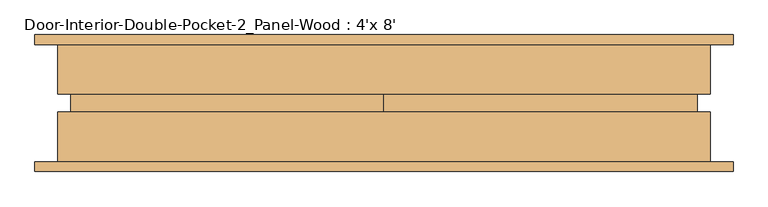
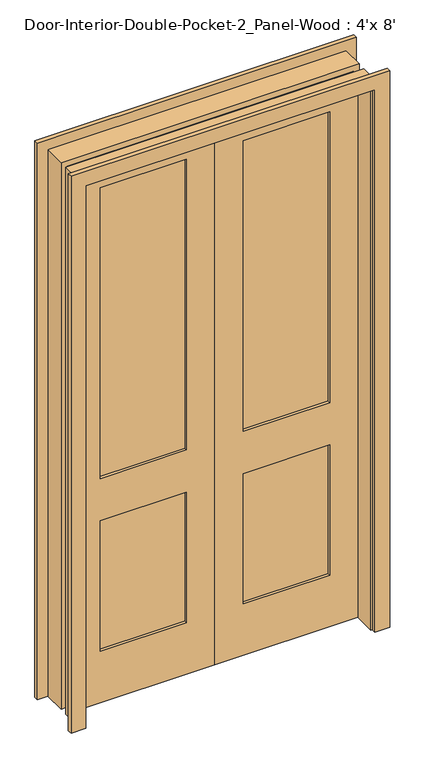
"""IFC4 building model written with IfcOpenShell, lengths in millimetres: door geometry, Door-Interior-Double-Pocket-2_Panel-Wood : 4'x 8'."""

from ifc_helpers import new_model, si_unit, frame, origin, place, context, project, spatial, polyline, outline, extrude, source, transform, mapped, element, save


def door_interior_double_pocket_2_panel_wood_4_x_8_12c354ae(model_context):
    return source(origin(), model_context, "Body", "SweptSolid", [
        extrude(outline(polyline([(0.0, 615.95), (0.0, 679.45), (2508.25, 679.45), (2508.25, -679.45), (0.0, -679.45), (0.0, -615.95), (2444.75, -615.95), (2444.75, 615.95), (0.0, 615.95)])), frame((0.0, 114.3, 0.0), z_axis=(0.0, 1.0, 0.0), x_axis=(0.0, 0.0, 1.0)), (0.0, 0.0, 1.0), 19.05),
        extrude(outline(polyline([(0.0, 615.95), (0.0, 679.45), (2508.25, 679.45), (2508.25, -679.45), (0.0, -679.45), (0.0, -615.95), (2444.75, -615.95), (2444.75, 615.95), (0.0, 615.95)])), frame((0.0, -133.35, 0.0), z_axis=(0.0, 1.0, 0.0), x_axis=(0.0, 0.0, 1.0)), (0.0, 0.0, 1.0), 19.05),
        extrude(outline(polyline([(2438.4, 0.0), (0.0, 0.0), (0.0, 609.6), (2438.4, 609.6), (2438.4, 0.0)]), holes=[polyline([(2319.3375, 120.65), (2319.3375, 488.95), (1009.65, 488.95), (1009.65, 120.65), (2319.3375, 120.65)]), polyline([(819.15, 120.65), (819.15, 488.95), (231.775, 488.95), (231.775, 120.65), (819.15, 120.65)])]), frame((0.0, -17.4625, 0.0), z_axis=(0.0, 1.0, 0.0), x_axis=(0.0, 0.0, 1.0)), (0.0, 0.0, 1.0), 34.925),
        extrude(outline(polyline([(488.95, -5.8208333), (120.65, -5.8208333), (120.65, 5.8208333), (488.95, 5.8208333), (488.95, -5.8208333)])), frame((0.0, 0.0, 1009.65), z_axis=(0.0, 0.0, 1.0), x_axis=(1.0, 0.0, 0.0)), (0.0, 0.0, 1.0), 1309.6875),
        extrude(outline(polyline([(488.95, -5.8208333), (120.65, -5.8208333), (120.65, 5.8208333), (488.95, 5.8208333), (488.95, -5.8208333)])), frame((0.0, 0.0, 231.775), z_axis=(0.0, 0.0, 1.0), x_axis=(1.0, 0.0, 0.0)), (0.0, 0.0, 1.0), 587.375),
        extrude(outline(polyline([(0.0, 635.0), (2463.8, 635.0), (2463.8, -635.0), (0.0, -635.0), (0.0, -609.6), (2438.4, -609.6), (2438.4, 609.6), (0.0, 609.6), (0.0, 635.0)])), frame((0.0, 17.4625, 0.0), z_axis=(0.0, 1.0, 0.0), x_axis=(0.0, 0.0, 1.0)), (0.0, 0.0, 1.0), 96.8375),
        extrude(outline(polyline([(0.0, 635.0), (2463.8, 635.0), (2463.8, -635.0), (0.0, -635.0), (0.0, -609.6), (2438.4, -609.6), (2438.4, 609.6), (0.0, 609.6), (0.0, 635.0)])), frame((0.0, -114.3, 0.0), z_axis=(0.0, 1.0, 0.0), x_axis=(0.0, 0.0, 1.0)), (0.0, 0.0, 1.0), 96.8375),
        extrude(outline(polyline([(2438.4, -609.6), (0.0, -609.6), (0.0, 0.0), (2438.4, 0.0), (2438.4, -609.6)]), holes=[polyline([(2319.3375, -488.95), (2319.3375, -120.65), (1009.65, -120.65), (1009.65, -488.95), (2319.3375, -488.95)]), polyline([(819.15, -488.95), (819.15, -120.65), (231.775, -120.65), (231.775, -488.95), (819.15, -488.95)])]), frame((0.0, -17.4625, 0.0), z_axis=(0.0, 1.0, 0.0), x_axis=(0.0, 0.0, 1.0)), (0.0, 0.0, 1.0), 34.925),
        extrude(outline(polyline([(-120.65, -5.8208333), (-488.95, -5.8208333), (-488.95, 5.8208333), (-120.65, 5.8208333), (-120.65, -5.8208333)])), frame((0.0, 0.0, 1009.65), z_axis=(0.0, 0.0, 1.0), x_axis=(1.0, 0.0, 0.0)), (0.0, 0.0, 1.0), 1309.6875),
        extrude(outline(polyline([(-120.65, -5.8208333), (-488.95, -5.8208333), (-488.95, 5.8208333), (-120.65, 5.8208333), (-120.65, -5.8208333)])), frame((0.0, 0.0, 231.775), z_axis=(0.0, 0.0, 1.0), x_axis=(1.0, 0.0, 0.0)), (0.0, 0.0, 1.0), 587.375),
    ])


if __name__ == "__main__":
    model = new_model("IFC4")
    model_context = context("Model", 3, world=origin())
    ifc_project = project(units=[si_unit("LENGTHUNIT", "METRE", prefix="MILLI")], contexts=[model_context])
    site = spatial("IfcSite", under=ifc_project)
    building = spatial("IfcBuilding", under=site)
    placement = place(None, origin())
    door_interior_double_pocket_2_panel_wood_4_x_8_shape = door_interior_double_pocket_2_panel_wood_4_x_8_12c354ae(model_context)
    element("IfcDoor", 1, ObjectType="Door-Interior-Double-Pocket-2_Panel-Wood : 4'x 8'", at=placement, inside=building, context=model_context, shape_type="MappedRepresentation", body=[
        mapped(door_interior_double_pocket_2_panel_wood_4_x_8_shape, transform((0.0, 0.0, 0.0), x_axis=(1.0, 0.0, 0.0), y_axis=(0.0, 1.0, 0.0), z_axis=(0.0, 0.0, 1.0))),
    ])
    save(model, "model.ifc")

# Revit data of these elements
# Type "Door-Interior-Double-Pocket-2_Panel-Wood : 4'x 8'"
#   Type Mark = "9"
#   Assembly Code = "C1020300"
#   Analytic Construction = "Wooden"
#   Top Rail = 0' - 4 11/16"
#   Thickness = 0' - 1 3/8"
#   Thermal Resistance (R) = 2.5876 (h·ft²·°F)/BTU
#   Stiles = 0' - 4 3/4"
#   Rough Width = 8' - 2"
#   Rough Height = 8' - 4 1/2"
#   Panel Width = 2' - 0"
#   Lock Rail = 0' - 7 1/2"
#   Location [instance default] = 2' - 1"
#   Height = 8' - 0"
#   Width = 4' - 0"
#   Heat Transfer Coefficient (U) = 0.3865 BTU/(h·ft²·°F)
#   Bottom Rail = 0' - 9 1/8"
#   Panel Open [instance default] = no
#   Trim Material = Cherry
#   Panel Material = wood door
#   Frame Material = Cherry
#   Visual Light Transmittance = 0
#   Solar Heat Gain Coefficient = 0
#   Wall Closure = (empty or 0)
#   Function = (empty or 0)
# Element 1 (IfcDoor, "Door-Interior-Double-Pocket-2_Panel-Wood : 4'x 8'")
#   Materials on its faces: "wood door", "Cherry"
# Materials
#   "Cherry": class "Wood", colour RGB 226 177 128, transparency 0, Description = "Prunus Serotina", Cost = 0
#   "wood door": class "Generic", colour RGB 120 120 120, transparency 0, Cost = 0
